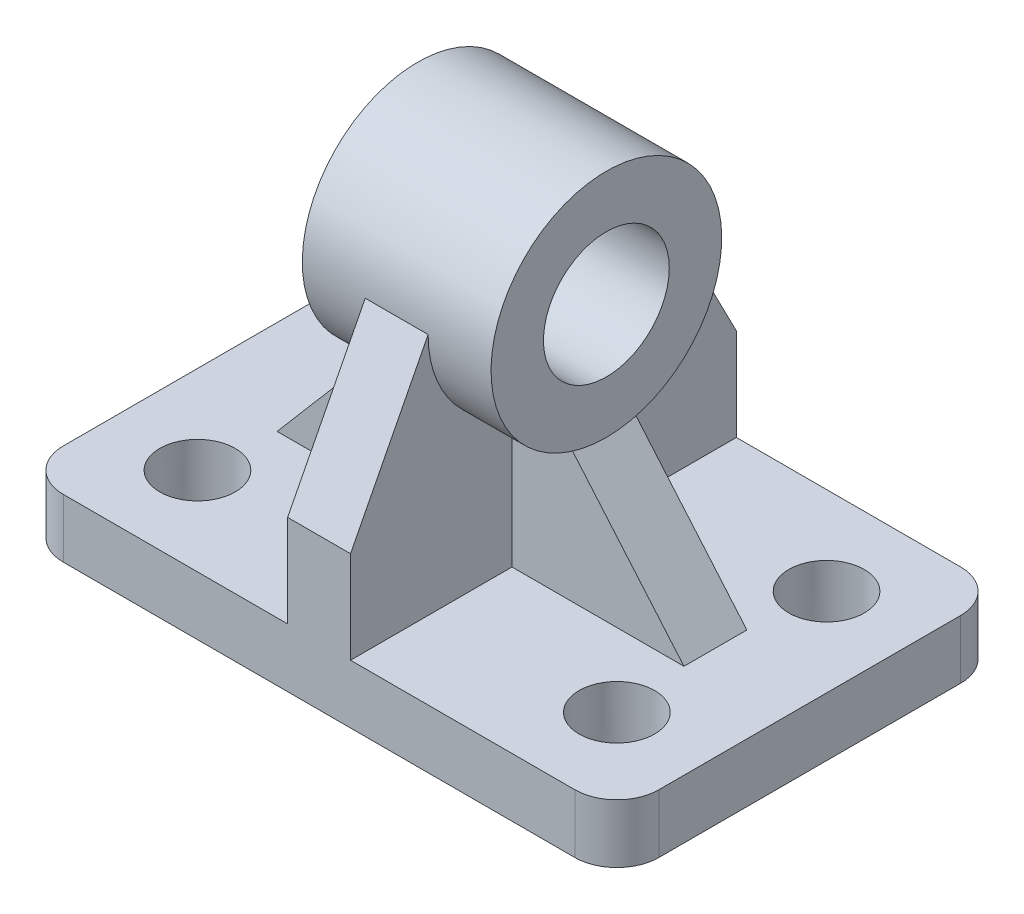
ISO-10303-21;
HEADER;
FILE_DESCRIPTION(('STEP AP214'),'2;1');
FILE_NAME('part.step','',(''),(''),'','','');
FILE_SCHEMA(('AUTOMOTIVE_DESIGN { 1 0 10303 214 1 1 1 1 }'));
ENDSEC;
DATA;
#1=APPLICATION_CONTEXT('core data for automotive mechanical design processes');
#2=APPLICATION_PROTOCOL_DEFINITION('international standard','automotive_design',2000,#1);
#3=PRODUCT_CONTEXT('',#1,'mechanical');
#4=PRODUCT('Part','Part','',(#3));
#5=PRODUCT_RELATED_PRODUCT_CATEGORY('part','',(#4));
#6=PRODUCT_DEFINITION_FORMATION('','',#4);
#7=PRODUCT_DEFINITION_CONTEXT('part definition',#1,'design');
#8=PRODUCT_DEFINITION('design','',#6,#7);
#9=PRODUCT_DEFINITION_SHAPE('','',#8);
#10=(LENGTH_UNIT() NAMED_UNIT(*) SI_UNIT(.MILLI.,.METRE.));
#11=(NAMED_UNIT(*) PLANE_ANGLE_UNIT() SI_UNIT($,.RADIAN.));
#12=(NAMED_UNIT(*) SI_UNIT($,.STERADIAN.) SOLID_ANGLE_UNIT());
#13=UNCERTAINTY_MEASURE_WITH_UNIT(LENGTH_MEASURE(1.E-05),#10,'distance_accuracy_value','');
#14=(GEOMETRIC_REPRESENTATION_CONTEXT(3) GLOBAL_UNCERTAINTY_ASSIGNED_CONTEXT((#13)) GLOBAL_UNIT_ASSIGNED_CONTEXT((#10,
#11,#12)) REPRESENTATION_CONTEXT('',''));
#15=CARTESIAN_POINT('',(0.,0.,0.));
#16=DIRECTION('',(0.,0.,1.));
#17=DIRECTION('',(1.,0.,0.));
#18=AXIS2_PLACEMENT_3D('',#15,#16,#17);
#19=CARTESIAN_POINT('',(-7.5,0.,0.));
#20=DIRECTION('',(1.,0.,0.));
#21=DIRECTION('',(0.,0.,-1.));
#22=AXIS2_PLACEMENT_3D('',#19,#20,#21);
#23=PLANE('',#22);
#24=DIRECTION('',(0.,-1.,0.));
#25=VECTOR('',#24,1.);
#26=CARTESIAN_POINT('',(-7.5,0.,-7.5));
#27=LINE('',#26,#25);
#28=CARTESIAN_POINT('',(-7.49999999999999,45.5423548405425,-7.5));
#29=VERTEX_POINT('',#28);
#30=CARTESIAN_POINT('',(-7.5,14.,-7.5));
#31=VERTEX_POINT('',#30);
#32=EDGE_CURVE('E215',#29,#31,#27,.T.);
#33=ORIENTED_EDGE('',*,*,#32,.F.);
#34=CARTESIAN_POINT('',(-7.5,72.,-0.000465840051602773));
#35=DIRECTION('',(1.,0.,0.));
#36=DIRECTION('',(0.,0.,-1.));
#37=AXIS2_PLACEMENT_3D('',#34,#35,#36);
#38=CIRCLE('',#37,27.5);
#39=CARTESIAN_POINT('',(-7.5,72.,-27.5004658400516));
#40=VERTEX_POINT('',#39);
#41=EDGE_CURVE('E11',#40,#29,#38,.F.);
#42=ORIENTED_EDGE('',*,*,#41,.F.);
#43=DIRECTION('',(0.,0.889435986634396,0.4570597616064));
#44=VECTOR('',#43,1.);
#45=CARTESIAN_POINT('',(-7.5,72.,-27.5004658400516));
#46=LINE('',#45,#44);
#47=CARTESIAN_POINT('',(-7.5,36.,-46.));
#48=VERTEX_POINT('',#47);
#49=EDGE_CURVE('E294',#48,#40,#46,.T.);
#50=ORIENTED_EDGE('',*,*,#49,.F.);
#51=DIRECTION('',(0.,1.,0.));
#52=VECTOR('',#51,1.);
#53=CARTESIAN_POINT('',(-7.5,14.,-46.));
#54=LINE('',#53,#52);
#55=CARTESIAN_POINT('',(-7.50000000000001,14.,-46.));
#56=VERTEX_POINT('',#55);
#57=EDGE_CURVE('E291',#56,#48,#54,.T.);
#58=ORIENTED_EDGE('',*,*,#57,.F.);
#59=DIRECTION('',(0.,0.,-1.));
#60=VECTOR('',#59,1.);
#61=CARTESIAN_POINT('',(-7.5,14.,46.));
#62=LINE('',#61,#60);
#63=EDGE_CURVE('E211',#31,#56,#62,.T.);
#64=ORIENTED_EDGE('',*,*,#63,.F.);
#65=EDGE_LOOP('',(#33,#42,#50,#58,#64));
#66=FACE_BOUND('',#65,.T.);
#67=ADVANCED_FACE('F44',(#66),#23,.F.);
#68=CARTESIAN_POINT('',(7.5,0.,0.));
#69=DIRECTION('',(1.,0.,0.));
#70=DIRECTION('',(0.,0.,-1.));
#71=AXIS2_PLACEMENT_3D('',#68,#69,#70);
#72=PLANE('',#71);
#73=CARTESIAN_POINT('',(7.5,72.,-0.000465840051602773));
#74=DIRECTION('',(1.,0.,0.));
#75=DIRECTION('',(0.,0.,-1.));
#76=AXIS2_PLACEMENT_3D('',#73,#74,#75);
#77=CIRCLE('',#76,27.5);
#78=CARTESIAN_POINT('',(7.5,72.,-27.5004658400516));
#79=VERTEX_POINT('',#78);
#80=CARTESIAN_POINT('',(7.5,45.5423548405425,-7.5));
#81=VERTEX_POINT('',#80);
#82=EDGE_CURVE('E274',#79,#81,#77,.F.);
#83=ORIENTED_EDGE('',*,*,#82,.T.);
#84=DIRECTION('',(0.,-1.,0.));
#85=VECTOR('',#84,1.);
#86=CARTESIAN_POINT('',(7.5,0.,-7.5));
#87=LINE('',#86,#85);
#88=CARTESIAN_POINT('',(7.5,14.,-7.5));
#89=VERTEX_POINT('',#88);
#90=EDGE_CURVE('E250',#81,#89,#87,.T.);
#91=ORIENTED_EDGE('',*,*,#90,.T.);
#92=DIRECTION('',(0.,0.,-1.));
#93=VECTOR('',#92,1.);
#94=CARTESIAN_POINT('',(7.5,14.,46.));
#95=LINE('',#94,#93);
#96=CARTESIAN_POINT('',(7.5,14.,-46.));
#97=VERTEX_POINT('',#96);
#98=EDGE_CURVE('E282',#89,#97,#95,.T.);
#99=ORIENTED_EDGE('',*,*,#98,.T.);
#100=DIRECTION('',(0.,1.,0.));
#101=VECTOR('',#100,1.);
#102=CARTESIAN_POINT('',(7.5,14.,-46.));
#103=LINE('',#102,#101);
#104=CARTESIAN_POINT('',(7.5,36.,-46.));
#105=VERTEX_POINT('',#104);
#106=EDGE_CURVE('E278',#97,#105,#103,.T.);
#107=ORIENTED_EDGE('',*,*,#106,.T.);
#108=DIRECTION('',(0.,0.889435986634396,0.4570597616064));
#109=VECTOR('',#108,1.);
#110=CARTESIAN_POINT('',(7.5,72.,-27.5004658400516));
#111=LINE('',#110,#109);
#112=EDGE_CURVE('E284',#105,#79,#111,.T.);
#113=ORIENTED_EDGE('',*,*,#112,.T.);
#114=EDGE_LOOP('',(#83,#91,#99,#107,#113));
#115=FACE_BOUND('',#114,.T.);
#116=ADVANCED_FACE('F414',(#115),#72,.T.);
#117=CARTESIAN_POINT('',(0.,14.,0.));
#118=DIRECTION('',(0.,-1.,0.));
#119=DIRECTION('',(0.,0.,-1.));
#120=AXIS2_PLACEMENT_3D('',#117,#118,#119);
#121=PLANE('',#120);
#122=CARTESIAN_POINT('',(50.,14.,25.));
#123=DIRECTION('',(0.,1.,0.));
#124=DIRECTION('',(0.,0.,1.));
#125=AXIS2_PLACEMENT_3D('',#122,#123,#124);
#126=CIRCLE('',#125,9.);
#127=CARTESIAN_POINT('',(50.,14.,34.));
#128=VERTEX_POINT('',#127);
#129=EDGE_CURVE('E554',#128,#128,#126,.T.);
#130=ORIENTED_EDGE('',*,*,#129,.F.);
#131=EDGE_LOOP('',(#130));
#132=FACE_BOUND('',#131,.T.);
#133=CARTESIAN_POINT('',(50.,14.,-25.));
#134=DIRECTION('',(0.,1.,0.));
#135=DIRECTION('',(0.,0.,1.));
#136=AXIS2_PLACEMENT_3D('',#133,#134,#135);
#137=CIRCLE('',#136,9.);
#138=CARTESIAN_POINT('',(50.,14.,-16.));
#139=VERTEX_POINT('',#138);
#140=EDGE_CURVE('E552',#139,#139,#137,.T.);
#141=ORIENTED_EDGE('',*,*,#140,.F.);
#142=EDGE_LOOP('',(#141));
#143=FACE_BOUND('',#142,.T.);
#144=DIRECTION('',(0.,0.,-1.));
#145=VECTOR('',#144,1.);
#146=CARTESIAN_POINT('',(71.,14.,46.));
#147=LINE('',#146,#145);
#148=CARTESIAN_POINT('',(71.,14.,36.));
#149=VERTEX_POINT('',#148);
#150=CARTESIAN_POINT('',(71.,14.,-36.));
#151=VERTEX_POINT('',#150);
#152=EDGE_CURVE('E315',#149,#151,#147,.T.);
#153=ORIENTED_EDGE('',*,*,#152,.T.);
#154=CARTESIAN_POINT('',(61.,14.,-36.));
#155=DIRECTION('',(0.,-1.,0.));
#156=DIRECTION('',(0.,0.,-1.));
#157=AXIS2_PLACEMENT_3D('',#154,#155,#156);
#158=CIRCLE('',#157,10.);
#159=CARTESIAN_POINT('',(61.,14.,-46.));
#160=VERTEX_POINT('',#159);
#161=EDGE_CURVE('E359',#151,#160,#158,.F.);
#162=ORIENTED_EDGE('',*,*,#161,.T.);
#163=DIRECTION('',(-1.,0.,0.));
#164=VECTOR('',#163,1.);
#165=CARTESIAN_POINT('',(-71.,14.,-46.));
#166=LINE('',#165,#164);
#167=EDGE_CURVE('E317',#160,#97,#166,.T.);
#168=ORIENTED_EDGE('',*,*,#167,.T.);
#169=ORIENTED_EDGE('',*,*,#98,.F.);
#170=DIRECTION('',(-1.,0.,0.));
#171=VECTOR('',#170,1.);
#172=CARTESIAN_POINT('',(0.,14.,-7.5));
#173=LINE('',#172,#171);
#174=CARTESIAN_POINT('',(48.5,14.,-7.5));
#175=VERTEX_POINT('',#174);
#176=EDGE_CURVE('E248',#175,#89,#173,.T.);
#177=ORIENTED_EDGE('',*,*,#176,.F.);
#178=DIRECTION('',(0.,0.,-1.));
#179=VECTOR('',#178,1.);
#180=CARTESIAN_POINT('',(48.5,14.,0.));
#181=LINE('',#180,#179);
#182=CARTESIAN_POINT('',(48.5,14.,7.5));
#183=VERTEX_POINT('',#182);
#184=EDGE_CURVE('E265',#175,#183,#181,.F.);
#185=ORIENTED_EDGE('',*,*,#184,.T.);
#186=DIRECTION('',(-1.,0.,0.));
#187=VECTOR('',#186,1.);
#188=CARTESIAN_POINT('',(0.,14.,7.5));
#189=LINE('',#188,#187);
#190=CARTESIAN_POINT('',(7.5,14.,7.5));
#191=VERTEX_POINT('',#190);
#192=EDGE_CURVE('E260',#183,#191,#189,.T.);
#193=ORIENTED_EDGE('',*,*,#192,.T.);
#194=CARTESIAN_POINT('',(7.50000000000001,14.,46.));
#195=VERTEX_POINT('',#194);
#196=EDGE_CURVE('E280',#195,#191,#95,.T.);
#197=ORIENTED_EDGE('',*,*,#196,.F.);
#198=DIRECTION('',(1.,0.,0.));
#199=VECTOR('',#198,1.);
#200=CARTESIAN_POINT('',(-71.,14.,46.));
#201=LINE('',#200,#199);
#202=CARTESIAN_POINT('',(61.,14.,46.));
#203=VERTEX_POINT('',#202);
#204=EDGE_CURVE('E322',#195,#203,#201,.T.);
#205=ORIENTED_EDGE('',*,*,#204,.T.);
#206=CARTESIAN_POINT('',(61.,14.,36.));
#207=DIRECTION('',(0.,-1.,0.));
#208=DIRECTION('',(0.,0.,-1.));
#209=AXIS2_PLACEMENT_3D('',#206,#207,#208);
#210=CIRCLE('',#209,10.);
#211=EDGE_CURVE('E354',#203,#149,#210,.F.);
#212=ORIENTED_EDGE('',*,*,#211,.T.);
#213=EDGE_LOOP('',(#153,#162,#168,#169,#177,#185,#193,#197,#205,#212));
#214=FACE_BOUND('',#213,.T.);
#215=ADVANCED_FACE('F423',(#132,#143,#214),#121,.F.);
#216=CARTESIAN_POINT('',(71.,14.,46.));
#217=DIRECTION('',(-1.,0.,0.));
#218=DIRECTION('',(0.,0.,1.));
#219=AXIS2_PLACEMENT_3D('',#216,#217,#218);
#220=PLANE('',#219);
#221=DIRECTION('',(0.,0.,-1.));
#222=VECTOR('',#221,1.);
#223=CARTESIAN_POINT('',(71.,0.,46.));
#224=LINE('',#223,#222);
#225=CARTESIAN_POINT('',(71.,0.,36.));
#226=VERTEX_POINT('',#225);
#227=CARTESIAN_POINT('',(71.,0.,-36.));
#228=VERTEX_POINT('',#227);
#229=EDGE_CURVE('E311',#226,#228,#224,.T.);
#230=ORIENTED_EDGE('',*,*,#229,.T.);
#231=DIRECTION('',(0.,-1.,0.));
#232=VECTOR('',#231,1.);
#233=CARTESIAN_POINT('',(71.,14.,-36.));
#234=LINE('',#233,#232);
#235=EDGE_CURVE('E353',#228,#151,#234,.F.);
#236=ORIENTED_EDGE('',*,*,#235,.T.);
#237=ORIENTED_EDGE('',*,*,#152,.F.);
#238=DIRECTION('',(0.,-1.,0.));
#239=VECTOR('',#238,1.);
#240=CARTESIAN_POINT('',(71.,14.,36.));
#241=LINE('',#240,#239);
#242=EDGE_CURVE('E349',#149,#226,#241,.T.);
#243=ORIENTED_EDGE('',*,*,#242,.T.);
#244=EDGE_LOOP('',(#230,#236,#237,#243));
#245=FACE_BOUND('',#244,.T.);
#246=ADVANCED_FACE('F510',(#245),#220,.F.);
#247=CARTESIAN_POINT('',(-71.,14.,-46.));
#248=DIRECTION('',(0.,0.,1.));
#249=DIRECTION('',(1.,0.,0.));
#250=AXIS2_PLACEMENT_3D('',#247,#248,#249);
#251=PLANE('',#250);
#252=ORIENTED_EDGE('',*,*,#167,.F.);
#253=DIRECTION('',(0.,-1.,0.));
#254=VECTOR('',#253,1.);
#255=CARTESIAN_POINT('',(61.,14.,-46.));
#256=LINE('',#255,#254);
#257=CARTESIAN_POINT('',(61.,0.,-46.));
#258=VERTEX_POINT('',#257);
#259=EDGE_CURVE('E332',#160,#258,#256,.T.);
#260=ORIENTED_EDGE('',*,*,#259,.T.);
#261=DIRECTION('',(-1.,0.,0.));
#262=VECTOR('',#261,1.);
#263=CARTESIAN_POINT('',(-71.,0.,-46.));
#264=LINE('',#263,#262);
#265=CARTESIAN_POINT('',(-61.,0.,-46.));
#266=VERTEX_POINT('',#265);
#267=EDGE_CURVE('E327',#258,#266,#264,.T.);
#268=ORIENTED_EDGE('',*,*,#267,.T.);
#269=DIRECTION('',(0.,-1.,0.));
#270=VECTOR('',#269,1.);
#271=CARTESIAN_POINT('',(-61.,14.,-46.));
#272=LINE('',#271,#270);
#273=CARTESIAN_POINT('',(-61.,14.,-46.));
#274=VERTEX_POINT('',#273);
#275=EDGE_CURVE('E321',#266,#274,#272,.F.);
#276=ORIENTED_EDGE('',*,*,#275,.T.);
#277=EDGE_CURVE('E313',#56,#274,#166,.T.);
#278=ORIENTED_EDGE('',*,*,#277,.F.);
#279=ORIENTED_EDGE('',*,*,#57,.T.);
#280=DIRECTION('',(-1.,0.,0.));
#281=VECTOR('',#280,1.);
#282=CARTESIAN_POINT('',(7.5,36.,-46.));
#283=LINE('',#282,#281);
#284=EDGE_CURVE('E308',#105,#48,#283,.T.);
#285=ORIENTED_EDGE('',*,*,#284,.F.);
#286=ORIENTED_EDGE('',*,*,#106,.F.);
#287=EDGE_LOOP('',(#252,#260,#268,#276,#278,#279,#285,#286));
#288=FACE_BOUND('',#287,.T.);
#289=ADVANCED_FACE('F481',(#288),#251,.F.);
#290=CARTESIAN_POINT('',(-71.,14.,46.));
#291=DIRECTION('',(1.,0.,0.));
#292=DIRECTION('',(0.,0.,-1.));
#293=AXIS2_PLACEMENT_3D('',#290,#291,#292);
#294=PLANE('',#293);
#295=DIRECTION('',(0.,-1.,0.));
#296=VECTOR('',#295,1.);
#297=CARTESIAN_POINT('',(-71.,14.,36.));
#298=LINE('',#297,#296);
#299=CARTESIAN_POINT('',(-71.,0.,36.));
#300=VERTEX_POINT('',#299);
#301=CARTESIAN_POINT('',(-71.,14.,36.));
#302=VERTEX_POINT('',#301);
#303=EDGE_CURVE('E365',#300,#302,#298,.F.);
#304=ORIENTED_EDGE('',*,*,#303,.T.);
#305=DIRECTION('',(0.,0.,1.));
#306=VECTOR('',#305,1.);
#307=CARTESIAN_POINT('',(-71.,14.,46.));
#308=LINE('',#307,#306);
#309=CARTESIAN_POINT('',(-71.,14.,-36.));
#310=VERTEX_POINT('',#309);
#311=EDGE_CURVE('E316',#310,#302,#308,.T.);
#312=ORIENTED_EDGE('',*,*,#311,.F.);
#313=DIRECTION('',(0.,-1.,0.));
#314=VECTOR('',#313,1.);
#315=CARTESIAN_POINT('',(-71.,14.,-36.));
#316=LINE('',#315,#314);
#317=CARTESIAN_POINT('',(-71.,0.,-36.));
#318=VERTEX_POINT('',#317);
#319=EDGE_CURVE('E362',#310,#318,#316,.T.);
#320=ORIENTED_EDGE('',*,*,#319,.T.);
#321=DIRECTION('',(0.,0.,1.));
#322=VECTOR('',#321,1.);
#323=CARTESIAN_POINT('',(-71.,0.,46.));
#324=LINE('',#323,#322);
#325=EDGE_CURVE('E326',#318,#300,#324,.T.);
#326=ORIENTED_EDGE('',*,*,#325,.T.);
#327=EDGE_LOOP('',(#304,#312,#320,#326));
#328=FACE_BOUND('',#327,.T.);
#329=ADVANCED_FACE('F493',(#328),#294,.F.);
#330=CARTESIAN_POINT('',(-71.,14.,46.));
#331=DIRECTION('',(0.,0.,-1.));
#332=DIRECTION('',(-1.,0.,0.));
#333=AXIS2_PLACEMENT_3D('',#330,#331,#332);
#334=PLANE('',#333);
#335=CARTESIAN_POINT('',(-61.,14.,46.));
#336=VERTEX_POINT('',#335);
#337=CARTESIAN_POINT('',(-7.50000000000001,14.,46.));
#338=VERTEX_POINT('',#337);
#339=EDGE_CURVE('E325',#336,#338,#201,.T.);
#340=ORIENTED_EDGE('',*,*,#339,.F.);
#341=DIRECTION('',(0.,-1.,0.));
#342=VECTOR('',#341,1.);
#343=CARTESIAN_POINT('',(-61.,14.,46.));
#344=LINE('',#343,#342);
#345=CARTESIAN_POINT('',(-61.,0.,46.));
#346=VERTEX_POINT('',#345);
#347=EDGE_CURVE('E371',#336,#346,#344,.T.);
#348=ORIENTED_EDGE('',*,*,#347,.T.);
#349=DIRECTION('',(1.,0.,0.));
#350=VECTOR('',#349,1.);
#351=CARTESIAN_POINT('',(-71.,0.,46.));
#352=LINE('',#351,#350);
#353=CARTESIAN_POINT('',(61.,0.,46.));
#354=VERTEX_POINT('',#353);
#355=EDGE_CURVE('E314',#346,#354,#352,.T.);
#356=ORIENTED_EDGE('',*,*,#355,.T.);
#357=DIRECTION('',(0.,-1.,0.));
#358=VECTOR('',#357,1.);
#359=CARTESIAN_POINT('',(61.,14.,46.));
#360=LINE('',#359,#358);
#361=EDGE_CURVE('E368',#354,#203,#360,.F.);
#362=ORIENTED_EDGE('',*,*,#361,.T.);
#363=ORIENTED_EDGE('',*,*,#204,.F.);
#364=DIRECTION('',(0.,-1.,0.));
#365=VECTOR('',#364,1.);
#366=CARTESIAN_POINT('',(7.5,14.,46.));
#367=LINE('',#366,#365);
#368=CARTESIAN_POINT('',(7.5,36.,46.));
#369=VERTEX_POINT('',#368);
#370=EDGE_CURVE('E290',#369,#195,#367,.T.);
#371=ORIENTED_EDGE('',*,*,#370,.F.);
#372=DIRECTION('',(-1.,0.,0.));
#373=VECTOR('',#372,1.);
#374=CARTESIAN_POINT('',(7.5,36.,46.));
#375=LINE('',#374,#373);
#376=CARTESIAN_POINT('',(-7.5,36.,46.));
#377=VERTEX_POINT('',#376);
#378=EDGE_CURVE('E287',#369,#377,#375,.T.);
#379=ORIENTED_EDGE('',*,*,#378,.T.);
#380=DIRECTION('',(0.,-1.,0.));
#381=VECTOR('',#380,1.);
#382=CARTESIAN_POINT('',(-7.5,14.,46.));
#383=LINE('',#382,#381);
#384=EDGE_CURVE('E299',#377,#338,#383,.T.);
#385=ORIENTED_EDGE('',*,*,#384,.T.);
#386=EDGE_LOOP('',(#340,#348,#356,#362,#363,#371,#379,#385));
#387=FACE_BOUND('',#386,.T.);
#388=ADVANCED_FACE('F517',(#387),#334,.F.);
#389=CARTESIAN_POINT('',(-50.,14.,25.));
#390=DIRECTION('',(0.,1.,0.));
#391=DIRECTION('',(0.,0.,1.));
#392=AXIS2_PLACEMENT_3D('',#389,#390,#391);
#393=CIRCLE('',#392,9.);
#394=CARTESIAN_POINT('',(-50.,14.,34.));
#395=VERTEX_POINT('',#394);
#396=EDGE_CURVE('E546',#395,#395,#393,.T.);
#397=ORIENTED_EDGE('',*,*,#396,.F.);
#398=EDGE_LOOP('',(#397));
#399=FACE_BOUND('',#398,.T.);
#400=CARTESIAN_POINT('',(-50.,14.,-25.));
#401=DIRECTION('',(0.,1.,0.));
#402=DIRECTION('',(0.,0.,1.));
#403=AXIS2_PLACEMENT_3D('',#400,#401,#402);
#404=CIRCLE('',#403,9.);
#405=CARTESIAN_POINT('',(-50.,14.,-16.));
#406=VERTEX_POINT('',#405);
#407=EDGE_CURVE('E379',#406,#406,#404,.T.);
#408=ORIENTED_EDGE('',*,*,#407,.F.);
#409=EDGE_LOOP('',(#408));
#410=FACE_BOUND('',#409,.T.);
#411=CARTESIAN_POINT('',(-7.5,14.,7.5));
#412=VERTEX_POINT('',#411);
#413=EDGE_CURVE('E293',#338,#412,#62,.T.);
#414=ORIENTED_EDGE('',*,*,#413,.T.);
#415=DIRECTION('',(-1.,0.,0.));
#416=VECTOR('',#415,1.);
#417=CARTESIAN_POINT('',(0.,14.,7.5));
#418=LINE('',#417,#416);
#419=CARTESIAN_POINT('',(-48.5,14.,7.5));
#420=VERTEX_POINT('',#419);
#421=EDGE_CURVE('E65',#412,#420,#418,.T.);
#422=ORIENTED_EDGE('',*,*,#421,.T.);
#423=DIRECTION('',(0.,0.,-1.));
#424=VECTOR('',#423,1.);
#425=CARTESIAN_POINT('',(-48.5,14.,0.));
#426=LINE('',#425,#424);
#427=CARTESIAN_POINT('',(-48.5,14.,-7.5));
#428=VERTEX_POINT('',#427);
#429=EDGE_CURVE('E67',#420,#428,#426,.T.);
#430=ORIENTED_EDGE('',*,*,#429,.T.);
#431=DIRECTION('',(-1.,0.,0.));
#432=VECTOR('',#431,1.);
#433=CARTESIAN_POINT('',(0.,14.,-7.5));
#434=LINE('',#433,#432);
#435=EDGE_CURVE('E217',#31,#428,#434,.T.);
#436=ORIENTED_EDGE('',*,*,#435,.F.);
#437=ORIENTED_EDGE('',*,*,#63,.T.);
#438=ORIENTED_EDGE('',*,*,#277,.T.);
#439=CARTESIAN_POINT('',(-61.,14.,-36.));
#440=DIRECTION('',(0.,-1.,0.));
#441=DIRECTION('',(0.,0.,-1.));
#442=AXIS2_PLACEMENT_3D('',#439,#440,#441);
#443=CIRCLE('',#442,10.);
#444=EDGE_CURVE('E356',#274,#310,#443,.F.);
#445=ORIENTED_EDGE('',*,*,#444,.T.);
#446=ORIENTED_EDGE('',*,*,#311,.T.);
#447=CARTESIAN_POINT('',(-61.,14.,36.));
#448=DIRECTION('',(0.,-1.,0.));
#449=DIRECTION('',(0.,0.,-1.));
#450=AXIS2_PLACEMENT_3D('',#447,#448,#449);
#451=CIRCLE('',#450,10.);
#452=EDGE_CURVE('E358',#302,#336,#451,.F.);
#453=ORIENTED_EDGE('',*,*,#452,.T.);
#454=ORIENTED_EDGE('',*,*,#339,.T.);
#455=EDGE_LOOP('',(#414,#422,#430,#436,#437,#438,#445,#446,#453,#454));
#456=FACE_BOUND('',#455,.T.);
#457=ADVANCED_FACE('F488',(#399,#410,#456),#121,.F.);
#458=CARTESIAN_POINT('',(0.,0.,0.));
#459=DIRECTION('',(0.,-1.,0.));
#460=DIRECTION('',(0.,0.,-1.));
#461=AXIS2_PLACEMENT_3D('',#458,#459,#460);
#462=PLANE('',#461);
#463=CARTESIAN_POINT('',(-50.,0.,25.));
#464=DIRECTION('',(0.,-1.,0.));
#465=DIRECTION('',(0.,0.,-1.));
#466=AXIS2_PLACEMENT_3D('',#463,#464,#465);
#467=CIRCLE('',#466,9.);
#468=CARTESIAN_POINT('',(-50.,0.,16.));
#469=VERTEX_POINT('',#468);
#470=EDGE_CURVE('E47',#469,#469,#467,.T.);
#471=ORIENTED_EDGE('',*,*,#470,.F.);
#472=EDGE_LOOP('',(#471));
#473=FACE_BOUND('',#472,.T.);
#474=CARTESIAN_POINT('',(50.,0.,25.));
#475=DIRECTION('',(0.,-1.,0.));
#476=DIRECTION('',(0.,0.,-1.));
#477=AXIS2_PLACEMENT_3D('',#474,#475,#476);
#478=CIRCLE('',#477,9.);
#479=CARTESIAN_POINT('',(50.,0.,16.));
#480=VERTEX_POINT('',#479);
#481=EDGE_CURVE('E385',#480,#480,#478,.T.);
#482=ORIENTED_EDGE('',*,*,#481,.F.);
#483=EDGE_LOOP('',(#482));
#484=FACE_BOUND('',#483,.T.);
#485=CARTESIAN_POINT('',(50.,0.,-25.));
#486=DIRECTION('',(0.,-1.,0.));
#487=DIRECTION('',(0.,0.,-1.));
#488=AXIS2_PLACEMENT_3D('',#485,#486,#487);
#489=CIRCLE('',#488,9.);
#490=CARTESIAN_POINT('',(50.,0.,-34.));
#491=VERTEX_POINT('',#490);
#492=EDGE_CURVE('E378',#491,#491,#489,.T.);
#493=ORIENTED_EDGE('',*,*,#492,.F.);
#494=EDGE_LOOP('',(#493));
#495=FACE_BOUND('',#494,.T.);
#496=CARTESIAN_POINT('',(-50.,0.,-25.));
#497=DIRECTION('',(0.,-1.,0.));
#498=DIRECTION('',(0.,0.,-1.));
#499=AXIS2_PLACEMENT_3D('',#496,#497,#498);
#500=CIRCLE('',#499,9.);
#501=CARTESIAN_POINT('',(-50.,0.,-34.));
#502=VERTEX_POINT('',#501);
#503=EDGE_CURVE('E376',#502,#502,#500,.T.);
#504=ORIENTED_EDGE('',*,*,#503,.F.);
#505=EDGE_LOOP('',(#504));
#506=FACE_BOUND('',#505,.T.);
#507=CARTESIAN_POINT('',(61.,0.,-36.));
#508=DIRECTION('',(0.,-1.,0.));
#509=DIRECTION('',(0.,0.,-1.));
#510=AXIS2_PLACEMENT_3D('',#507,#508,#509);
#511=CIRCLE('',#510,10.);
#512=EDGE_CURVE('E343',#258,#228,#511,.T.);
#513=ORIENTED_EDGE('',*,*,#512,.T.);
#514=ORIENTED_EDGE('',*,*,#229,.F.);
#515=CARTESIAN_POINT('',(61.,0.,36.));
#516=DIRECTION('',(0.,-1.,0.));
#517=DIRECTION('',(0.,0.,-1.));
#518=AXIS2_PLACEMENT_3D('',#515,#516,#517);
#519=CIRCLE('',#518,10.);
#520=EDGE_CURVE('E336',#226,#354,#519,.T.);
#521=ORIENTED_EDGE('',*,*,#520,.T.);
#522=ORIENTED_EDGE('',*,*,#355,.F.);
#523=CARTESIAN_POINT('',(-61.,0.,36.));
#524=DIRECTION('',(0.,-1.,0.));
#525=DIRECTION('',(0.,0.,-1.));
#526=AXIS2_PLACEMENT_3D('',#523,#524,#525);
#527=CIRCLE('',#526,10.);
#528=EDGE_CURVE('E338',#346,#300,#527,.T.);
#529=ORIENTED_EDGE('',*,*,#528,.T.);
#530=ORIENTED_EDGE('',*,*,#325,.F.);
#531=CARTESIAN_POINT('',(-61.,0.,-36.));
#532=DIRECTION('',(0.,-1.,0.));
#533=DIRECTION('',(0.,0.,-1.));
#534=AXIS2_PLACEMENT_3D('',#531,#532,#533);
#535=CIRCLE('',#534,10.);
#536=EDGE_CURVE('E344',#318,#266,#535,.T.);
#537=ORIENTED_EDGE('',*,*,#536,.T.);
#538=ORIENTED_EDGE('',*,*,#267,.F.);
#539=EDGE_LOOP('',(#513,#514,#521,#522,#529,#530,#537,#538));
#540=FACE_BOUND('',#539,.T.);
#541=ADVANCED_FACE('F498',(#473,#484,#495,#506,#540),#462,.T.);
#542=CARTESIAN_POINT('',(61.,14.,-36.));
#543=DIRECTION('',(0.,-1.,0.));
#544=DIRECTION('',(0.,0.,-1.));
#545=AXIS2_PLACEMENT_3D('',#542,#543,#544);
#546=CYLINDRICAL_SURFACE('',#545,10.);
#547=ORIENTED_EDGE('',*,*,#161,.F.);
#548=ORIENTED_EDGE('',*,*,#235,.F.);
#549=ORIENTED_EDGE('',*,*,#512,.F.);
#550=ORIENTED_EDGE('',*,*,#259,.F.);
#551=EDGE_LOOP('',(#547,#548,#549,#550));
#552=FACE_BOUND('',#551,.T.);
#553=ADVANCED_FACE('F505',(#552),#546,.T.);
#554=CARTESIAN_POINT('',(-61.,14.,-36.));
#555=DIRECTION('',(0.,-1.,0.));
#556=DIRECTION('',(0.,0.,-1.));
#557=AXIS2_PLACEMENT_3D('',#554,#555,#556);
#558=CYLINDRICAL_SURFACE('',#557,10.);
#559=ORIENTED_EDGE('',*,*,#444,.F.);
#560=ORIENTED_EDGE('',*,*,#275,.F.);
#561=ORIENTED_EDGE('',*,*,#536,.F.);
#562=ORIENTED_EDGE('',*,*,#319,.F.);
#563=EDGE_LOOP('',(#559,#560,#561,#562));
#564=FACE_BOUND('',#563,.T.);
#565=ADVANCED_FACE('F492',(#564),#558,.T.);
#566=CARTESIAN_POINT('',(-61.,14.,36.));
#567=DIRECTION('',(0.,-1.,0.));
#568=DIRECTION('',(0.,0.,-1.));
#569=AXIS2_PLACEMENT_3D('',#566,#567,#568);
#570=CYLINDRICAL_SURFACE('',#569,10.);
#571=ORIENTED_EDGE('',*,*,#452,.F.);
#572=ORIENTED_EDGE('',*,*,#303,.F.);
#573=ORIENTED_EDGE('',*,*,#528,.F.);
#574=ORIENTED_EDGE('',*,*,#347,.F.);
#575=EDGE_LOOP('',(#571,#572,#573,#574));
#576=FACE_BOUND('',#575,.T.);
#577=ADVANCED_FACE('F518',(#576),#570,.T.);
#578=CARTESIAN_POINT('',(61.,14.,36.));
#579=DIRECTION('',(0.,-1.,0.));
#580=DIRECTION('',(0.,0.,-1.));
#581=AXIS2_PLACEMENT_3D('',#578,#579,#580);
#582=CYLINDRICAL_SURFACE('',#581,10.);
#583=ORIENTED_EDGE('',*,*,#211,.F.);
#584=ORIENTED_EDGE('',*,*,#361,.F.);
#585=ORIENTED_EDGE('',*,*,#520,.F.);
#586=ORIENTED_EDGE('',*,*,#242,.F.);
#587=EDGE_LOOP('',(#583,#584,#585,#586));
#588=FACE_BOUND('',#587,.T.);
#589=ADVANCED_FACE('F50',(#588),#582,.T.);
#590=CARTESIAN_POINT('',(7.5,72.,-27.5004658400516));
#591=DIRECTION('',(0.,-0.4570597616064,0.889435986634396));
#592=DIRECTION('',(0.,-0.889435986634396,-0.4570597616064));
#593=AXIS2_PLACEMENT_3D('',#590,#591,#592);
#594=PLANE('',#593);
#595=ORIENTED_EDGE('',*,*,#49,.T.);
#596=DIRECTION('',(-1.,0.,0.));
#597=VECTOR('',#596,1.);
#598=CARTESIAN_POINT('',(7.5,72.,-27.5004658400516));
#599=LINE('',#598,#597);
#600=EDGE_CURVE('E207',#79,#40,#599,.T.);
#601=ORIENTED_EDGE('',*,*,#600,.F.);
#602=ORIENTED_EDGE('',*,*,#112,.F.);
#603=ORIENTED_EDGE('',*,*,#284,.T.);
#604=EDGE_LOOP('',(#595,#601,#602,#603));
#605=FACE_BOUND('',#604,.T.);
#606=ADVANCED_FACE('F476',(#605),#594,.F.);
#607=CARTESIAN_POINT('',(7.5,72.,27.4995341599484));
#608=DIRECTION('',(0.,-0.45707797125468,-0.889426628898475));
#609=DIRECTION('',(0.,0.889426628898475,-0.45707797125468));
#610=AXIS2_PLACEMENT_3D('',#607,#608,#609);
#611=PLANE('',#610);
#612=DIRECTION('',(0.,-0.889426628898475,0.45707797125468));
#613=VECTOR('',#612,1.);
#614=CARTESIAN_POINT('',(-7.5,72.,27.4995341599484));
#615=LINE('',#614,#613);
#616=CARTESIAN_POINT('',(-7.5,72.,27.4995341599484));
#617=VERTEX_POINT('',#616);
#618=EDGE_CURVE('E300',#617,#377,#615,.T.);
#619=ORIENTED_EDGE('',*,*,#618,.T.);
#620=ORIENTED_EDGE('',*,*,#378,.F.);
#621=DIRECTION('',(0.,-0.889426628898475,0.45707797125468));
#622=VECTOR('',#621,1.);
#623=CARTESIAN_POINT('',(7.5,72.,27.4995341599484));
#624=LINE('',#623,#622);
#625=CARTESIAN_POINT('',(7.5,72.,27.4995341599484));
#626=VERTEX_POINT('',#625);
#627=EDGE_CURVE('E283',#626,#369,#624,.T.);
#628=ORIENTED_EDGE('',*,*,#627,.F.);
#629=DIRECTION('',(-1.,0.,0.));
#630=VECTOR('',#629,1.);
#631=CARTESIAN_POINT('',(7.5,72.,27.4995341599484));
#632=LINE('',#631,#630);
#633=EDGE_CURVE('E302',#626,#617,#632,.T.);
#634=ORIENTED_EDGE('',*,*,#633,.T.);
#635=EDGE_LOOP('',(#619,#620,#628,#634));
#636=FACE_BOUND('',#635,.T.);
#637=ADVANCED_FACE('F435',(#636),#611,.F.);
#638=DIRECTION('',(0.,-1.,0.));
#639=VECTOR('',#638,1.);
#640=CARTESIAN_POINT('',(7.5,0.,7.5));
#641=LINE('',#640,#639);
#642=CARTESIAN_POINT('',(7.5,45.5426189470269,7.5));
#643=VERTEX_POINT('',#642);
#644=EDGE_CURVE('E251',#643,#191,#641,.T.);
#645=ORIENTED_EDGE('',*,*,#644,.F.);
#646=EDGE_CURVE('E267',#643,#626,#77,.F.);
#647=ORIENTED_EDGE('',*,*,#646,.T.);
#648=ORIENTED_EDGE('',*,*,#627,.T.);
#649=ORIENTED_EDGE('',*,*,#370,.T.);
#650=ORIENTED_EDGE('',*,*,#196,.T.);
#651=EDGE_LOOP('',(#645,#647,#648,#649,#650));
#652=FACE_BOUND('',#651,.T.);
#653=ADVANCED_FACE('F425',(#652),#72,.T.);
#654=CARTESIAN_POINT('',(-7.5,45.5426189470269,7.5));
#655=VERTEX_POINT('',#654);
#656=EDGE_CURVE('E53',#655,#617,#38,.F.);
#657=ORIENTED_EDGE('',*,*,#656,.F.);
#658=DIRECTION('',(0.,-1.,0.));
#659=VECTOR('',#658,1.);
#660=CARTESIAN_POINT('',(-7.5,0.,7.5));
#661=LINE('',#660,#659);
#662=EDGE_CURVE('E233',#655,#412,#661,.T.);
#663=ORIENTED_EDGE('',*,*,#662,.T.);
#664=ORIENTED_EDGE('',*,*,#413,.F.);
#665=ORIENTED_EDGE('',*,*,#384,.F.);
#666=ORIENTED_EDGE('',*,*,#618,.F.);
#667=EDGE_LOOP('',(#657,#663,#664,#665,#666));
#668=FACE_BOUND('',#667,.T.);
#669=ADVANCED_FACE('F413',(#668),#23,.F.);
#670=CARTESIAN_POINT('',(22.5,72.,-0.000465840051602773));
#671=DIRECTION('',(-1.,0.,0.));
#672=DIRECTION('',(0.,0.,1.));
#673=AXIS2_PLACEMENT_3D('',#670,#671,#672);
#674=CYLINDRICAL_SURFACE('',#673,27.5);
#675=CARTESIAN_POINT('',(-0.94262295081966,72.,-0.000465840051602773));
#676=DIRECTION('',(-0.761015091093203,-0.648734176013878,0.));
#677=DIRECTION('',(-0.648734176013878,0.761015091093203,0.));
#678=AXIS2_PLACEMENT_3D('',#675,#676,#677);
#679=ELLIPSE('',#678,36.1359456886671,27.5);
#680=CARTESIAN_POINT('',(22.5,44.5,-0.000465840051602773));
#681=VERTEX_POINT('',#680);
#682=CARTESIAN_POINT('',(21.6114352178982,45.5423548405425,-7.5));
#683=VERTEX_POINT('',#682);
#684=EDGE_CURVE('E256',#681,#683,#679,.F.);
#685=ORIENTED_EDGE('',*,*,#684,.T.);
#686=DIRECTION('',(-1.,0.,0.));
#687=VECTOR('',#686,1.);
#688=CARTESIAN_POINT('',(22.5,45.5423548405425,-7.5));
#689=LINE('',#688,#687);
#690=EDGE_CURVE('E245',#81,#683,#689,.F.);
#691=ORIENTED_EDGE('',*,*,#690,.F.);
#692=ORIENTED_EDGE('',*,*,#82,.F.);
#693=ORIENTED_EDGE('',*,*,#600,.T.);
#694=ORIENTED_EDGE('',*,*,#41,.T.);
#695=DIRECTION('',(-1.,0.,0.));
#696=VECTOR('',#695,1.);
#697=CARTESIAN_POINT('',(22.5,45.5423548405425,-7.5));
#698=LINE('',#697,#696);
#699=CARTESIAN_POINT('',(-21.6114352178982,45.5423548405425,-7.5));
#700=VERTEX_POINT('',#699);
#701=EDGE_CURVE('E205',#700,#29,#698,.F.);
#702=ORIENTED_EDGE('',*,*,#701,.F.);
#703=CARTESIAN_POINT('',(0.942622950819712,72.,-0.000465840051602773));
#704=DIRECTION('',(-0.761015091093202,0.648734176013878,0.));
#705=DIRECTION('',(-0.648734176013878,-0.761015091093202,0.));
#706=AXIS2_PLACEMENT_3D('',#703,#704,#705);
#707=ELLIPSE('',#706,36.1359456886671,27.5);
#708=CARTESIAN_POINT('',(-22.5,44.5,-0.000465840051602773));
#709=VERTEX_POINT('',#708);
#710=EDGE_CURVE('E234',#700,#709,#707,.T.);
#711=ORIENTED_EDGE('',*,*,#710,.T.);
#712=CARTESIAN_POINT('',(-22.5,72.,-0.000465840051602773));
#713=DIRECTION('',(1.,0.,0.));
#714=DIRECTION('',(0.,0.,-1.));
#715=AXIS2_PLACEMENT_3D('',#712,#713,#714);
#716=CIRCLE('',#715,27.5);
#717=EDGE_CURVE('E272',#709,#709,#716,.T.);
#718=ORIENTED_EDGE('',*,*,#717,.T.);
#719=CARTESIAN_POINT('',(-21.6112100779442,45.5426189470269,7.5));
#720=VERTEX_POINT('',#719);
#721=EDGE_CURVE('E236',#709,#720,#707,.T.);
#722=ORIENTED_EDGE('',*,*,#721,.T.);
#723=DIRECTION('',(-1.,0.,0.));
#724=VECTOR('',#723,1.);
#725=CARTESIAN_POINT('',(22.5,45.5426189470269,7.5));
#726=LINE('',#725,#724);
#727=EDGE_CURVE('E230',#720,#655,#726,.F.);
#728=ORIENTED_EDGE('',*,*,#727,.T.);
#729=ORIENTED_EDGE('',*,*,#656,.T.);
#730=ORIENTED_EDGE('',*,*,#633,.F.);
#731=ORIENTED_EDGE('',*,*,#646,.F.);
#732=DIRECTION('',(-1.,0.,0.));
#733=VECTOR('',#732,1.);
#734=CARTESIAN_POINT('',(22.5,45.5426189470269,7.5));
#735=LINE('',#734,#733);
#736=CARTESIAN_POINT('',(21.6112100779443,45.5426189470269,7.5));
#737=VERTEX_POINT('',#736);
#738=EDGE_CURVE('E255',#643,#737,#735,.F.);
#739=ORIENTED_EDGE('',*,*,#738,.T.);
#740=EDGE_CURVE('E262',#737,#681,#679,.F.);
#741=ORIENTED_EDGE('',*,*,#740,.T.);
#742=CARTESIAN_POINT('',(22.5,72.,-0.000465840051602773));
#743=DIRECTION('',(1.,0.,0.));
#744=DIRECTION('',(0.,0.,-1.));
#745=AXIS2_PLACEMENT_3D('',#742,#743,#744);
#746=CIRCLE('',#745,27.5);
#747=EDGE_CURVE('E266',#681,#681,#746,.T.);
#748=ORIENTED_EDGE('',*,*,#747,.F.);
#749=EDGE_LOOP('',(#685,#691,#692,#693,#694,#702,#711,#718,#722,#728,#729,#730,#731,#739,#741,#748));
#750=FACE_BOUND('',#749,.T.);
#751=ADVANCED_FACE('F198',(#750),#674,.T.);
#752=CARTESIAN_POINT('',(22.5,72.,-0.000465840051602773));
#753=DIRECTION('',(1.,0.,0.));
#754=DIRECTION('',(0.,0.,-1.));
#755=AXIS2_PLACEMENT_3D('',#752,#753,#754);
#756=PLANE('',#755);
#757=CARTESIAN_POINT('',(22.5,72.,-0.000465840051602773));
#758=DIRECTION('',(1.,0.,0.));
#759=DIRECTION('',(0.,0.,-1.));
#760=AXIS2_PLACEMENT_3D('',#757,#758,#759);
#761=CIRCLE('',#760,15.);
#762=CARTESIAN_POINT('',(22.5,72.,-15.0004658400516));
#763=VERTEX_POINT('',#762);
#764=EDGE_CURVE('E261',#763,#763,#761,.T.);
#765=ORIENTED_EDGE('',*,*,#764,.F.);
#766=EDGE_LOOP('',(#765));
#767=FACE_BOUND('',#766,.T.);
#768=ORIENTED_EDGE('',*,*,#747,.T.);
#769=EDGE_LOOP('',(#768));
#770=FACE_BOUND('',#769,.T.);
#771=ADVANCED_FACE('F399',(#767,#770),#756,.T.);
#772=CARTESIAN_POINT('',(-22.5,72.,-0.000465840051602773));
#773=DIRECTION('',(1.,0.,0.));
#774=DIRECTION('',(0.,0.,-1.));
#775=AXIS2_PLACEMENT_3D('',#772,#773,#774);
#776=PLANE('',#775);
#777=CARTESIAN_POINT('',(-22.5,72.,-0.000465840051602773));
#778=DIRECTION('',(1.,0.,0.));
#779=DIRECTION('',(0.,0.,-1.));
#780=AXIS2_PLACEMENT_3D('',#777,#778,#779);
#781=CIRCLE('',#780,15.);
#782=CARTESIAN_POINT('',(-22.5,72.,-15.0004658400516));
#783=VERTEX_POINT('',#782);
#784=EDGE_CURVE('E270',#783,#783,#781,.T.);
#785=ORIENTED_EDGE('',*,*,#784,.T.);
#786=EDGE_LOOP('',(#785));
#787=FACE_BOUND('',#786,.T.);
#788=ORIENTED_EDGE('',*,*,#717,.F.);
#789=EDGE_LOOP('',(#788));
#790=FACE_BOUND('',#789,.T.);
#791=ADVANCED_FACE('F398',(#787,#790),#776,.F.);
#792=CARTESIAN_POINT('',(-71.,72.,-0.000465840051602773));
#793=DIRECTION('',(1.,0.,0.));
#794=DIRECTION('',(0.,0.,-1.));
#795=AXIS2_PLACEMENT_3D('',#792,#793,#794);
#796=CYLINDRICAL_SURFACE('',#795,15.);
#797=ORIENTED_EDGE('',*,*,#764,.T.);
#798=EDGE_LOOP('',(#797));
#799=FACE_BOUND('',#798,.T.);
#800=ORIENTED_EDGE('',*,*,#784,.F.);
#801=EDGE_LOOP('',(#800));
#802=FACE_BOUND('',#801,.T.);
#803=ADVANCED_FACE('F396',(#799,#802),#796,.F.);
#804=CARTESIAN_POINT('',(22.5,44.5,0.));
#805=DIRECTION('',(-0.761015091093203,-0.648734176013878,0.));
#806=DIRECTION('',(0.648734176013877,-0.761015091093203,0.));
#807=AXIS2_PLACEMENT_3D('',#804,#805,#806);
#808=PLANE('',#807);
#809=ORIENTED_EDGE('',*,*,#184,.F.);
#810=DIRECTION('',(0.648734176013877,-0.761015091093203,0.));
#811=VECTOR('',#810,1.);
#812=CARTESIAN_POINT('',(22.5,44.5,-7.5));
#813=LINE('',#812,#811);
#814=EDGE_CURVE('E238',#683,#175,#813,.T.);
#815=ORIENTED_EDGE('',*,*,#814,.F.);
#816=ORIENTED_EDGE('',*,*,#684,.F.);
#817=ORIENTED_EDGE('',*,*,#740,.F.);
#818=DIRECTION('',(0.648734176013877,-0.761015091093203,0.));
#819=VECTOR('',#818,1.);
#820=CARTESIAN_POINT('',(22.5,44.5,7.5));
#821=LINE('',#820,#819);
#822=EDGE_CURVE('E237',#737,#183,#821,.T.);
#823=ORIENTED_EDGE('',*,*,#822,.T.);
#824=EDGE_LOOP('',(#809,#815,#816,#817,#823));
#825=FACE_BOUND('',#824,.T.);
#826=ADVANCED_FACE('F407',(#825),#808,.F.);
#827=CARTESIAN_POINT('',(0.,49.75,7.5));
#828=DIRECTION('',(0.,0.,1.));
#829=DIRECTION('',(1.,0.,0.));
#830=AXIS2_PLACEMENT_3D('',#827,#828,#829);
#831=PLANE('',#830);
#832=ORIENTED_EDGE('',*,*,#192,.F.);
#833=ORIENTED_EDGE('',*,*,#822,.F.);
#834=ORIENTED_EDGE('',*,*,#738,.F.);
#835=ORIENTED_EDGE('',*,*,#644,.T.);
#836=EDGE_LOOP('',(#832,#833,#834,#835));
#837=FACE_BOUND('',#836,.T.);
#838=ADVANCED_FACE('F453',(#837),#831,.T.);
#839=CARTESIAN_POINT('',(0.,49.75,-7.5));
#840=DIRECTION('',(0.,0.,1.));
#841=DIRECTION('',(1.,0.,0.));
#842=AXIS2_PLACEMENT_3D('',#839,#840,#841);
#843=PLANE('',#842);
#844=ORIENTED_EDGE('',*,*,#814,.T.);
#845=ORIENTED_EDGE('',*,*,#176,.T.);
#846=ORIENTED_EDGE('',*,*,#90,.F.);
#847=ORIENTED_EDGE('',*,*,#690,.T.);
#848=EDGE_LOOP('',(#844,#845,#846,#847));
#849=FACE_BOUND('',#848,.T.);
#850=ADVANCED_FACE('F448',(#849),#843,.F.);
#851=CARTESIAN_POINT('',(-22.5,44.5,0.));
#852=DIRECTION('',(-0.761015091093202,0.648734176013878,0.));
#853=DIRECTION('',(-0.648734176013878,-0.761015091093202,0.));
#854=AXIS2_PLACEMENT_3D('',#851,#852,#853);
#855=PLANE('',#854);
#856=ORIENTED_EDGE('',*,*,#429,.F.);
#857=DIRECTION('',(-0.648734176013878,-0.761015091093202,0.));
#858=VECTOR('',#857,1.);
#859=CARTESIAN_POINT('',(-22.5,44.5,7.5));
#860=LINE('',#859,#858);
#861=EDGE_CURVE('E225',#720,#420,#860,.T.);
#862=ORIENTED_EDGE('',*,*,#861,.F.);
#863=ORIENTED_EDGE('',*,*,#721,.F.);
#864=ORIENTED_EDGE('',*,*,#710,.F.);
#865=DIRECTION('',(-0.648734176013878,-0.761015091093202,0.));
#866=VECTOR('',#865,1.);
#867=CARTESIAN_POINT('',(-22.5,44.5,-7.5));
#868=LINE('',#867,#866);
#869=EDGE_CURVE('E223',#700,#428,#868,.T.);
#870=ORIENTED_EDGE('',*,*,#869,.T.);
#871=EDGE_LOOP('',(#856,#862,#863,#864,#870));
#872=FACE_BOUND('',#871,.T.);
#873=ADVANCED_FACE('F388',(#872),#855,.T.);
#874=CARTESIAN_POINT('',(0.,49.75,7.5));
#875=DIRECTION('',(0.,0.,1.));
#876=DIRECTION('',(1.,0.,0.));
#877=AXIS2_PLACEMENT_3D('',#874,#875,#876);
#878=PLANE('',#877);
#879=ORIENTED_EDGE('',*,*,#421,.F.);
#880=ORIENTED_EDGE('',*,*,#662,.F.);
#881=ORIENTED_EDGE('',*,*,#727,.F.);
#882=ORIENTED_EDGE('',*,*,#861,.T.);
#883=EDGE_LOOP('',(#879,#880,#881,#882));
#884=FACE_BOUND('',#883,.T.);
#885=ADVANCED_FACE('F441',(#884),#878,.T.);
#886=CARTESIAN_POINT('',(0.,49.75,-7.5));
#887=DIRECTION('',(0.,0.,1.));
#888=DIRECTION('',(1.,0.,0.));
#889=AXIS2_PLACEMENT_3D('',#886,#887,#888);
#890=PLANE('',#889);
#891=ORIENTED_EDGE('',*,*,#32,.T.);
#892=ORIENTED_EDGE('',*,*,#435,.T.);
#893=ORIENTED_EDGE('',*,*,#869,.F.);
#894=ORIENTED_EDGE('',*,*,#701,.T.);
#895=EDGE_LOOP('',(#891,#892,#893,#894));
#896=FACE_BOUND('',#895,.T.);
#897=ADVANCED_FACE('F216',(#896),#890,.F.);
#898=CARTESIAN_POINT('',(-50.,-27.,-25.));
#899=DIRECTION('',(0.,1.,0.));
#900=DIRECTION('',(0.,0.,1.));
#901=AXIS2_PLACEMENT_3D('',#898,#899,#900);
#902=CYLINDRICAL_SURFACE('',#901,9.);
#903=ORIENTED_EDGE('',*,*,#503,.T.);
#904=EDGE_LOOP('',(#903));
#905=FACE_BOUND('',#904,.T.);
#906=ORIENTED_EDGE('',*,*,#407,.T.);
#907=EDGE_LOOP('',(#906));
#908=FACE_BOUND('',#907,.T.);
#909=ADVANCED_FACE('F449',(#905,#908),#902,.F.);
#910=CARTESIAN_POINT('',(50.,-27.,-25.));
#911=DIRECTION('',(0.,1.,0.));
#912=DIRECTION('',(0.,0.,1.));
#913=AXIS2_PLACEMENT_3D('',#910,#911,#912);
#914=CYLINDRICAL_SURFACE('',#913,9.);
#915=ORIENTED_EDGE('',*,*,#492,.T.);
#916=EDGE_LOOP('',(#915));
#917=FACE_BOUND('',#916,.T.);
#918=ORIENTED_EDGE('',*,*,#140,.T.);
#919=EDGE_LOOP('',(#918));
#920=FACE_BOUND('',#919,.T.);
#921=ADVANCED_FACE('F562',(#917,#920),#914,.F.);
#922=CARTESIAN_POINT('',(50.,-27.,25.));
#923=DIRECTION('',(0.,1.,0.));
#924=DIRECTION('',(0.,0.,1.));
#925=AXIS2_PLACEMENT_3D('',#922,#923,#924);
#926=CYLINDRICAL_SURFACE('',#925,9.);
#927=ORIENTED_EDGE('',*,*,#481,.T.);
#928=EDGE_LOOP('',(#927));
#929=FACE_BOUND('',#928,.T.);
#930=ORIENTED_EDGE('',*,*,#129,.T.);
#931=EDGE_LOOP('',(#930));
#932=FACE_BOUND('',#931,.T.);
#933=ADVANCED_FACE('F561',(#929,#932),#926,.F.);
#934=CARTESIAN_POINT('',(-50.,-27.,25.));
#935=DIRECTION('',(0.,1.,0.));
#936=DIRECTION('',(0.,0.,1.));
#937=AXIS2_PLACEMENT_3D('',#934,#935,#936);
#938=CYLINDRICAL_SURFACE('',#937,9.);
#939=ORIENTED_EDGE('',*,*,#470,.T.);
#940=EDGE_LOOP('',(#939));
#941=FACE_BOUND('',#940,.T.);
#942=ORIENTED_EDGE('',*,*,#396,.T.);
#943=EDGE_LOOP('',(#942));
#944=FACE_BOUND('',#943,.T.);
#945=ADVANCED_FACE('F563',(#941,#944),#938,.F.);
#946=CLOSED_SHELL('',(#67,#116,#215,#246,#289,#329,#388,#457,#541,#553,#565,#577,#589,#606,#637,
#653,#669,#751,#771,#791,#803,#826,#838,#850,#873,#885,#897,#909,#921,#933,#945));
#947=MANIFOLD_SOLID_BREP('B2',#946);
#948=ADVANCED_BREP_SHAPE_REPRESENTATION('',(#18,#947),#14);
#949=SHAPE_DEFINITION_REPRESENTATION(#9,#948);
ENDSEC;
END-ISO-10303-21;
